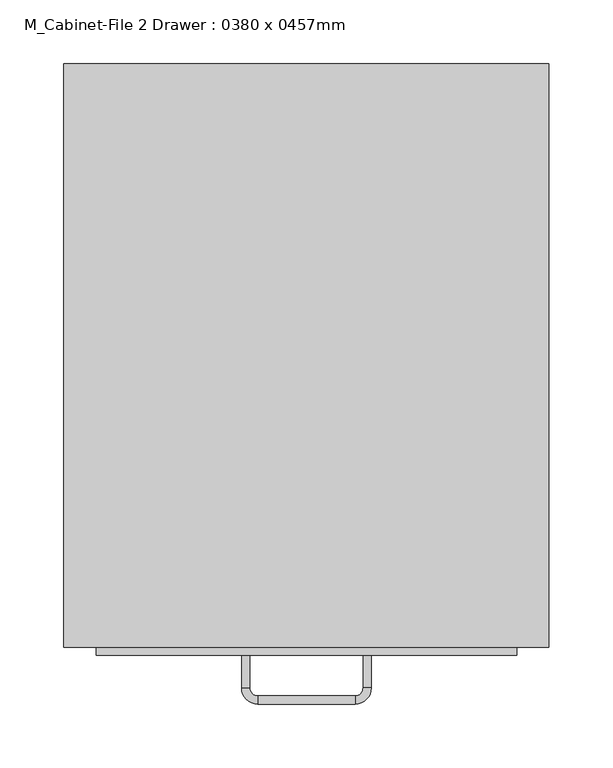
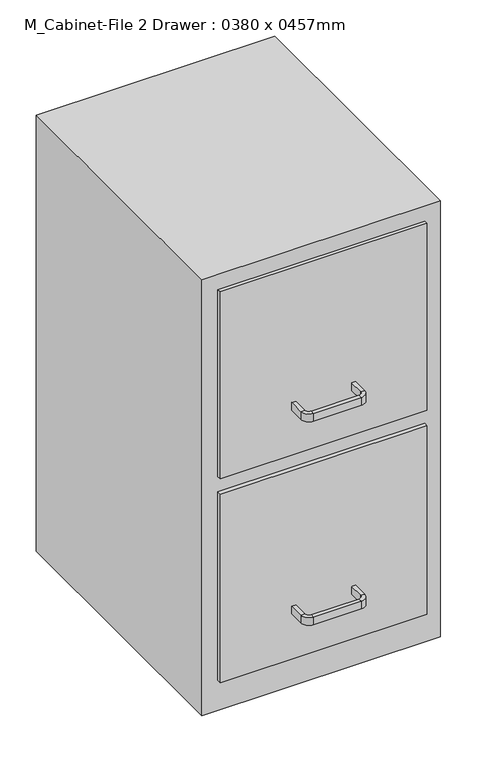
"""IFC4 building model written with IfcOpenShell, lengths in millimetres: furniture geometry, M_Cabinet-File 2 Drawer : 0380 x 0457mm."""

from ifc_helpers import new_model, si_unit, frame, origin, origin_with_axes, place, context, project, spatial, polyline, circle_curve, outline, extrude, source, transform, mapped, element, save
from ifc_brep_helpers import plane_surface, cylinder_surface, revolved_surface, advanced_brep


def m_cabinet_file_2_drawer_0380_x_0457mm_9eec7cff(model_context):
    return source(origin(), model_context, "Body", "SolidModel", [
        extrude(outline(polyline([(36.703553, -376.9843001), (-292.496447, -376.9843001), (-292.496447, -370.6343001), (36.703553, -370.6343001), (36.703553, -376.9843001)])), frame((0.0, 0.0, 393.7), z_axis=(0.0, 0.0, 1.0), x_axis=(1.0, 0.0, 0.0)), (0.0, 0.0, 1.0), 314.9),
        extrude(outline(polyline([(36.703553, -376.9843001), (-292.496447, -376.9843001), (-292.496447, -370.6343001), (36.703553, -370.6343001), (36.703553, -376.9843001)])), frame((0.0, 0.0, 50.8), z_axis=(0.0, 0.0, 1.0), x_axis=(1.0, 0.0, 0.0)), (0.0, 0.0, 1.0), 317.5),
        advanced_brep(
        [(-172.346447, -376.9843001, 127.0), (-178.696447, -376.9843001, 127.0), (-178.696447, -376.9843001, 139.7), (-172.346447, -376.9843001, 139.7), (-172.346447, -402.3843001, 127.0), (-178.696447, -402.3843001, 127.0), (-178.696447, -402.3843001, 139.7), (-172.346447, -402.3843001, 139.7), (-165.996447, -415.0843001, 127.0), (-165.996447, -408.7343001, 127.0), (-165.996447, -415.0843001, 139.7), (-165.996447, -408.7343001, 139.7), (-89.796447, -408.7343001, 127.0), (-89.796447, -415.0843001, 127.0), (-89.796447, -415.0843001, 139.7), (-89.796447, -408.7343001, 139.7), (-77.096447, -402.3843001, 127.0), (-83.446447, -402.3843001, 127.0), (-77.096447, -402.3843001, 139.7), (-83.446447, -402.3843001, 139.7), (-83.446447, -376.9843001, 127.0), (-83.446447, -376.9843001, 139.7), (-77.096447, -376.9843001, 139.7), (-77.096447, -376.9843001, 127.0)],
        [
            (0, 1),
            (1, 2),
            (2, 3),
            (3, 0),
            (0, 4),
            (4, 5),
            (5, 1),
            (5, 6),
            (6, 2),
            (6, 7),
            (7, 3),
            (7, 4),
            (8, 5, circle_curve(frame((-165.996447, -402.3843001, 127.0), z_axis=(0.0, 0.0, -1.0), x_axis=(-1.0, 0.0, 0.0)), 12.7)),
            (4, 9, circle_curve(frame((-165.996447, -402.3843001, 127.0), z_axis=(0.0, 0.0, 1.0), x_axis=(-1.0, 0.0, 0.0)), 6.35)),
            (9, 8),
            (10, 6, circle_curve(frame((-165.996447, -402.3843001, 139.7), z_axis=(0.0, 0.0, -1.0), x_axis=(-1.0, 0.0, 0.0)), 12.7)),
            (8, 10),
            (11, 7, circle_curve(frame((-165.996447, -402.3843001, 139.7), z_axis=(0.0, 0.0, -1.0), x_axis=(-1.0, 0.0, 0.0)), 6.35)),
            (10, 11),
            (11, 9),
            (9, 12),
            (12, 13),
            (13, 8),
            (13, 14),
            (14, 10),
            (14, 15),
            (15, 11),
            (15, 12),
            (16, 13, circle_curve(frame((-89.796447, -402.3843001, 127.0), z_axis=(0.0, 0.0, -1.0), x_axis=(0.0, -1.0, 0.0)), 12.7)),
            (12, 17, circle_curve(frame((-89.796447, -402.3843001, 127.0), z_axis=(0.0, 0.0, 1.0), x_axis=(0.0, -1.0, 0.0)), 6.35)),
            (17, 16),
            (18, 14, circle_curve(frame((-89.796447, -402.3843001, 139.7), z_axis=(0.0, 0.0, -1.0), x_axis=(0.0, -1.0, 0.0)), 12.7)),
            (16, 18),
            (19, 15, circle_curve(frame((-89.796447, -402.3843001, 139.7), z_axis=(0.0, 0.0, -1.0), x_axis=(0.0, -1.0, 0.0)), 6.35)),
            (18, 19),
            (19, 17),
            (20, 21),
            (21, 22),
            (22, 23),
            (23, 20),
            (17, 20),
            (23, 16),
            (22, 18),
            (21, 19),
        ],
        [
            plane_surface(frame((-661.3382215, -376.9843001, 0.0), z_axis=(0.0, 1.0, 0.0), x_axis=(0.0, 0.0, -1.0))),
            plane_surface(frame((-172.346447, -376.9843001, 127.0), z_axis=(0.0, 0.0, -1.0), x_axis=(0.0, -1.0, 0.0))),
            plane_surface(frame((-178.696447, -376.9843001, 127.0), z_axis=(-1.0, 0.0, 0.0), x_axis=(0.0, -1.0, 0.0))),
            plane_surface(frame((-178.696447, -376.9843001, 139.7), z_axis=(0.0, 0.0, 1.0), x_axis=(0.0, -1.0, 0.0))),
            plane_surface(frame((-172.346447, -376.9843001, 139.7), z_axis=(1.0, 0.0, 0.0), x_axis=(0.0, -1.0, 0.0))),
            plane_surface(frame((-165.996447, -402.3843001, 127.0), z_axis=(0.0, 0.0, -1.0), x_axis=(-1.0, 0.0, 0.0))),
            cylinder_surface(frame((-165.996447, -402.3843001, 0.0), z_axis=(0.0, 0.0, 1.0), x_axis=(-1.0, 0.0, 0.0)), 12.7),
            plane_surface(frame((-165.996447, -402.3843001, 139.7), z_axis=(0.0, 0.0, 1.0), x_axis=(-1.0, 0.0, 0.0))),
            revolved_surface(polyline([(-172.34644699999998, -402.3843001, 139.7), (-172.34644699999998, -402.3843001, 127.0)]), (-165.996447, -402.3843001, 0.0), (0.0, 0.0, 1.0)),
            plane_surface(frame((-165.996447, -408.7343001, 127.0), z_axis=(0.0, 0.0, -1.0), x_axis=(1.0, 0.0, 0.0))),
            plane_surface(frame((-165.996447, -415.0843001, 127.0), z_axis=(0.0, -1.0, 0.0), x_axis=(1.0, 0.0, 0.0))),
            plane_surface(frame((-165.996447, -415.0843001, 139.7), z_axis=(0.0, 0.0, 1.0), x_axis=(1.0, 0.0, 0.0))),
            plane_surface(frame((-165.996447, -408.7343001, 139.7), z_axis=(0.0, 1.0, 0.0), x_axis=(1.0, 0.0, 0.0))),
            plane_surface(frame((-89.796447, -402.3843001, 127.0), z_axis=(0.0, 0.0, -1.0), x_axis=(0.0, -1.0, 0.0))),
            cylinder_surface(frame((-89.796447, -402.3843001, 0.0), z_axis=(0.0, 0.0, 1.0), x_axis=(0.0, -1.0, 0.0)), 12.7),
            plane_surface(frame((-89.796447, -402.3843001, 139.7), z_axis=(0.0, 0.0, 1.0), x_axis=(0.0, -1.0, 0.0))),
            revolved_surface(polyline([(-89.796447, -408.73430010000004, 139.7), (-89.796447, -408.73430010000004, 127.0)]), (-89.796447, -402.3843001, 0.0), (0.0, 0.0, 1.0)),
            plane_surface(frame((-559.7382215, -376.9843001, 0.0), z_axis=(0.0, 1.0, 0.0), x_axis=(0.0, 0.0, 1.0))),
            plane_surface(frame((-83.446447, -402.3843001, 127.0), z_axis=(0.0, 0.0, -1.0), x_axis=(0.0, 1.0, 0.0))),
            plane_surface(frame((-77.096447, -402.3843001, 127.0), z_axis=(1.0, 0.0, 0.0), x_axis=(0.0, 1.0, 0.0))),
            plane_surface(frame((-77.096447, -402.3843001, 139.7), z_axis=(0.0, 0.0, 1.0), x_axis=(0.0, 1.0, 0.0))),
            plane_surface(frame((-83.446447, -402.3843001, 139.7), z_axis=(-1.0, 0.0, 0.0), x_axis=(0.0, 1.0, 0.0))),
        ],
        [
            (0, [[1, 2, 3, 4]]),
            (1, [[-1, 5, 6, 7]]),
            (2, [[-2, -7, 8, 9]]),
            (3, [[-3, -9, 10, 11]]),
            (4, [[-4, -11, 12, -5]]),
            (5, [[13, -6, 14, 15]]),
            (6, [[16, -8, -13, 17]]),
            (7, [[18, -10, -16, 19]]),
            (8, [[-14, -12, -18, 20]]),
            (9, [[-15, 21, 22, 23]]),
            (10, [[-17, -23, 24, 25]]),
            (11, [[-19, -25, 26, 27]]),
            (12, [[-20, -27, 28, -21]]),
            (13, [[29, -22, 30, 31]]),
            (14, [[32, -24, -29, 33]]),
            (15, [[34, -26, -32, 35]]),
            (16, [[-30, -28, -34, 36]]),
            (17, [[37, 38, 39, 40]]),
            (18, [[-31, 41, -40, 42]]),
            (19, [[-33, -42, -39, 43]]),
            (20, [[-35, -43, -38, 44]]),
            (21, [[-36, -44, -37, -41]]),
        ],
    ),
        advanced_brep(
        [(-172.346447, -376.9843001, 469.9), (-178.696447, -376.9843001, 469.9), (-178.696447, -376.9843001, 482.6), (-172.346447, -376.9843001, 482.6), (-172.346447, -402.3843001, 469.9), (-178.696447, -402.3843001, 469.9), (-178.696447, -402.3843001, 482.6), (-172.346447, -402.3843001, 482.6), (-165.996447, -415.0843001, 469.9), (-165.996447, -408.7343001, 469.9), (-165.996447, -415.0843001, 482.6), (-165.996447, -408.7343001, 482.6), (-89.796447, -408.7343001, 469.9), (-89.796447, -415.0843001, 469.9), (-89.796447, -415.0843001, 482.6), (-89.796447, -408.7343001, 482.6), (-77.096447, -402.3843001, 469.9), (-83.446447, -402.3843001, 469.9), (-77.096447, -402.3843001, 482.6), (-83.446447, -402.3843001, 482.6), (-83.446447, -376.9843001, 469.9), (-83.446447, -376.9843001, 482.6), (-77.096447, -376.9843001, 482.6), (-77.096447, -376.9843001, 469.9)],
        [
            (0, 1),
            (1, 2),
            (2, 3),
            (3, 0),
            (0, 4),
            (4, 5),
            (5, 1),
            (5, 6),
            (6, 2),
            (6, 7),
            (7, 3),
            (7, 4),
            (8, 5, circle_curve(frame((-165.996447, -402.3843001, 469.9), z_axis=(0.0, 0.0, -1.0), x_axis=(-1.0, 0.0, 0.0)), 12.7)),
            (4, 9, circle_curve(frame((-165.996447, -402.3843001, 469.9), z_axis=(0.0, 0.0, 1.0), x_axis=(-1.0, 0.0, 0.0)), 6.35)),
            (9, 8),
            (10, 6, circle_curve(frame((-165.996447, -402.3843001, 482.6), z_axis=(0.0, 0.0, -1.0), x_axis=(-1.0, 0.0, 0.0)), 12.7)),
            (8, 10),
            (11, 7, circle_curve(frame((-165.996447, -402.3843001, 482.6), z_axis=(0.0, 0.0, -1.0), x_axis=(-1.0, 0.0, 0.0)), 6.35)),
            (10, 11),
            (11, 9),
            (9, 12),
            (12, 13),
            (13, 8),
            (13, 14),
            (14, 10),
            (14, 15),
            (15, 11),
            (15, 12),
            (16, 13, circle_curve(frame((-89.796447, -402.3843001, 469.9), z_axis=(0.0, 0.0, -1.0), x_axis=(0.0, -1.0, 0.0)), 12.7)),
            (12, 17, circle_curve(frame((-89.796447, -402.3843001, 469.9), z_axis=(0.0, 0.0, 1.0), x_axis=(0.0, -1.0, 0.0)), 6.35)),
            (17, 16),
            (18, 14, circle_curve(frame((-89.796447, -402.3843001, 482.6), z_axis=(0.0, 0.0, -1.0), x_axis=(0.0, -1.0, 0.0)), 12.7)),
            (16, 18),
            (19, 15, circle_curve(frame((-89.796447, -402.3843001, 482.6), z_axis=(0.0, 0.0, -1.0), x_axis=(0.0, -1.0, 0.0)), 6.35)),
            (18, 19),
            (19, 17),
            (20, 21),
            (21, 22),
            (22, 23),
            (23, 20),
            (17, 20),
            (23, 16),
            (22, 18),
            (21, 19),
        ],
        [
            plane_surface(frame((-661.3382215, -376.9843001, 0.0), z_axis=(0.0, 1.0, 0.0), x_axis=(0.0, 0.0, -1.0))),
            plane_surface(frame((-172.346447, -376.9843001, 469.9), z_axis=(0.0, 0.0, -1.0), x_axis=(0.0, -1.0, 0.0))),
            plane_surface(frame((-178.696447, -376.9843001, 469.9), z_axis=(-1.0, 0.0, 0.0), x_axis=(0.0, -1.0, 0.0))),
            plane_surface(frame((-178.696447, -376.9843001, 482.6), z_axis=(0.0, 0.0, 1.0), x_axis=(0.0, -1.0, 0.0))),
            plane_surface(frame((-172.346447, -376.9843001, 482.6), z_axis=(1.0, 0.0, 0.0), x_axis=(0.0, -1.0, 0.0))),
            plane_surface(frame((-165.996447, -402.3843001, 469.9), z_axis=(0.0, 0.0, -1.0), x_axis=(-1.0, 0.0, 0.0))),
            cylinder_surface(frame((-165.996447, -402.3843001, 0.0), z_axis=(0.0, 0.0, 1.0), x_axis=(-1.0, 0.0, 0.0)), 12.7),
            plane_surface(frame((-165.996447, -402.3843001, 482.6), z_axis=(0.0, 0.0, 1.0), x_axis=(-1.0, 0.0, 0.0))),
            revolved_surface(polyline([(-172.34644699999998, -402.3843001, 482.6), (-172.34644699999998, -402.3843001, 469.9)]), (-165.996447, -402.3843001, 0.0), (0.0, 0.0, 1.0)),
            plane_surface(frame((-165.996447, -408.7343001, 469.9), z_axis=(0.0, 0.0, -1.0), x_axis=(1.0, 0.0, 0.0))),
            plane_surface(frame((-165.996447, -415.0843001, 469.9), z_axis=(0.0, -1.0, 0.0), x_axis=(1.0, 0.0, 0.0))),
            plane_surface(frame((-165.996447, -415.0843001, 482.6), z_axis=(0.0, 0.0, 1.0), x_axis=(1.0, 0.0, 0.0))),
            plane_surface(frame((-165.996447, -408.7343001, 482.6), z_axis=(0.0, 1.0, 0.0), x_axis=(1.0, 0.0, 0.0))),
            plane_surface(frame((-89.796447, -402.3843001, 469.9), z_axis=(0.0, 0.0, -1.0), x_axis=(0.0, -1.0, 0.0))),
            cylinder_surface(frame((-89.796447, -402.3843001, 0.0), z_axis=(0.0, 0.0, 1.0), x_axis=(0.0, -1.0, 0.0)), 12.7),
            plane_surface(frame((-89.796447, -402.3843001, 482.6), z_axis=(0.0, 0.0, 1.0), x_axis=(0.0, -1.0, 0.0))),
            revolved_surface(polyline([(-89.796447, -408.73430010000004, 482.6), (-89.796447, -408.73430010000004, 469.9)]), (-89.796447, -402.3843001, 0.0), (0.0, 0.0, 1.0)),
            plane_surface(frame((-559.7382215, -376.9843001, 0.0), z_axis=(0.0, 1.0, 0.0), x_axis=(0.0, 0.0, 1.0))),
            plane_surface(frame((-83.446447, -402.3843001, 469.9), z_axis=(0.0, 0.0, -1.0), x_axis=(0.0, 1.0, 0.0))),
            plane_surface(frame((-77.096447, -402.3843001, 469.9), z_axis=(1.0, 0.0, 0.0), x_axis=(0.0, 1.0, 0.0))),
            plane_surface(frame((-77.096447, -402.3843001, 482.6), z_axis=(0.0, 0.0, 1.0), x_axis=(0.0, 1.0, 0.0))),
            plane_surface(frame((-83.446447, -402.3843001, 482.6), z_axis=(-1.0, 0.0, 0.0), x_axis=(0.0, 1.0, 0.0))),
        ],
        [
            (0, [[1, 2, 3, 4]]),
            (1, [[-1, 5, 6, 7]]),
            (2, [[-2, -7, 8, 9]]),
            (3, [[-3, -9, 10, 11]]),
            (4, [[-4, -11, 12, -5]]),
            (5, [[13, -6, 14, 15]]),
            (6, [[16, -8, -13, 17]]),
            (7, [[18, -10, -16, 19]]),
            (8, [[-14, -12, -18, 20]]),
            (9, [[-15, 21, 22, 23]]),
            (10, [[-17, -23, 24, 25]]),
            (11, [[-19, -25, 26, 27]]),
            (12, [[-20, -27, 28, -21]]),
            (13, [[29, -22, 30, 31]]),
            (14, [[32, -24, -29, 33]]),
            (15, [[34, -26, -32, 35]]),
            (16, [[-30, -28, -34, 36]]),
            (17, [[37, 38, 39, 40]]),
            (18, [[-31, 41, -40, 42]]),
            (19, [[-33, -42, -39, 43]]),
            (20, [[-35, -43, -38, 44]]),
            (21, [[-36, -44, -37, -41]]),
        ],
    ),
        extrude(outline(polyline([(62.103553, 86.3656999), (62.103553, -370.6343001), (-317.896447, -370.6343001), (-317.896447, 86.3656999), (62.103553, 86.3656999)])), origin_with_axes(), (0.0, 0.0, 1.0), 734.0),
    ])


if __name__ == "__main__":
    model = new_model("IFC4")
    model_context = context("Model", 3, world=origin())
    ifc_project = project(units=[si_unit("LENGTHUNIT", "METRE", prefix="MILLI")], contexts=[model_context])
    site = spatial("IfcSite", under=ifc_project)
    building = spatial("IfcBuilding", under=site)
    placement = place(None, origin())
    m_cabinet_file_2_drawer_0380_x_0457mm_shape = m_cabinet_file_2_drawer_0380_x_0457mm_9eec7cff(model_context)
    element("IfcFurniture", 1, ObjectType="M_Cabinet-File 2 Drawer : 0380 x 0457mm", at=placement, inside=building, context=model_context, shape_type="MappedRepresentation", body=[
        mapped(m_cabinet_file_2_drawer_0380_x_0457mm_shape, transform((0.0, 0.0, 0.0), x_axis=(1.0, 0.0, 0.0), y_axis=(0.0, 1.0, 0.0), z_axis=(0.0, 0.0, 1.0))),
    ])
    save(model, "model.ifc")

# Revit data of these elements
# Type "M_Cabinet-File 2 Drawer : 0380 x 0457mm"
#   Depth = 457 mm
#   Height = 734 mm
#   Width = 380 mm
#   Cabinet Material = Steel, Paint Finish, Ivory, Glossy
#   Handle Material = Steel, Chrome Plated
#   Default Elevation = 0
# Element 1 (IfcFurniture, "M_Cabinet-File 2 Drawer : 0380 x 0457mm")
#   Materials on its faces: "Steel, Chrome Plated", "Steel, Paint Finish, Ivory, Glossy"
# Materials
#   "Steel, Paint Finish, Ivory, Glossy": class "Metal", colour RGB 247 247 239, transparency 0, Description = "Steel, paint finish, ivory, glossy", Cost = 0
#   "Steel, Chrome Plated": class "Metal", colour RGB 244 244 244, transparency 0, Description = "Chromiuim plated steel", Cost = 0
